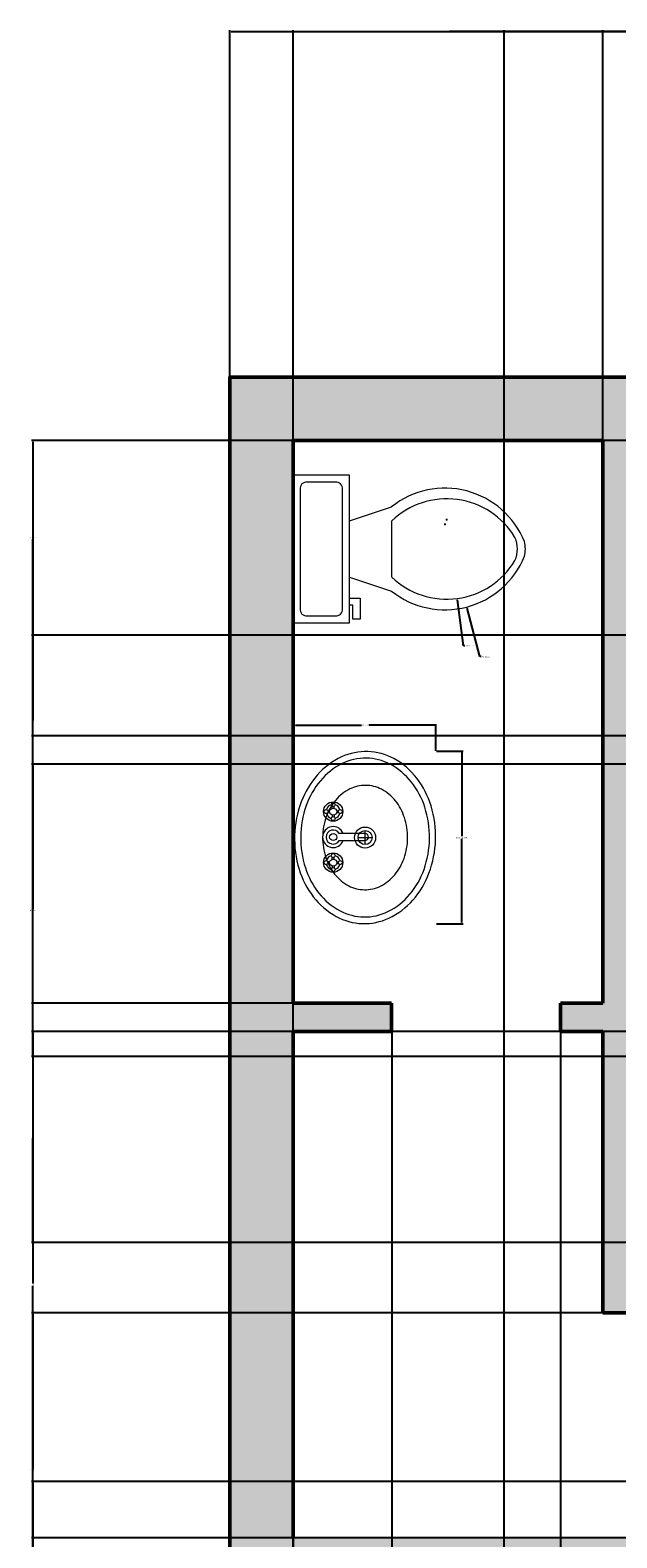
# Model space of a CAD drawing. Units: inches. Extents: x 1869 to 2483, y 2084 to 2479.
# Tile 3 of 7: x 1869 to 1952, y 2265 to 2479. Entities that reach past the tile are written whole.
import ezdxf

# ---------------------------------------------------------------- set-up
doc = ezdxf.new("R2010")
doc.units = ezdxf.units.IN
for name, color, linetype, lineweight in [('A-ANNO-DIMS', 2, 'Continuous', 18), ('A-FLOR-FIXT', 9, 'Continuous', 18), ('A-WALL', 7, 'Continuous', 50)]:
    doc.layers.add(name, color=color, linetype=linetype, lineweight=lineweight)
doc.layers.add('A-WALL-PATT', color=18, linetype='Continuous', lineweight=13, true_color=0x000000)
doc.styles.get("Standard").update_dxf_attribs({"font": 'arial.ttf'})
doc.dimstyles.get("Standard").update_dxf_attribs({"dimtxt": 0.18, "dimasz": 0.18, "dimexe": 0.18, "dimexo": 0.0625, "dimgap": 0.09, "dimtad": 0, "dimtih": 1, "dimtoh": 1, "dimdec": 4, "dimzin": 0, "dimdsep": 46, "dimtxsty": 'Standard', "dimcen": 0.09, "dimadec": 0, "dimazin": 0, "dimtfac": 1, "dimtdec": 4, "dimtofl": 0, "dimtmove": 0, "dimatfit": 3, "dimfxl": 1, "dimtolj": 1, "dimtzin": 0, "dimarcsym": 0})

# ---------------------------------------------------------------- blocks, each defined once
blk = doc.blocks.new('Toilet - top')
for p, q in [((9.5, -6), (9.5, -2)), ((-10, -8.5), (-8, -8.5)), ((-10, -9.5), (-10, -8.5)), ((-8, -8.5), (-8, -8)), ((-7, -8), (-7, -9.5)), ((-4, -8), (-6, -14)), ((4, -8), (6, -14)), ((-7, -9.5), (-10, -9.5)), ((4, -14), (-4, -14))]:
    blk.add_line(p, q)
blk.add_lwpolyline([(10.5, -8), (10.5, 0), (-10.5, 0), (-10.5, -8)], close=True)
for points in [[(-9.5, -2), (-9.5, -6)], [(8.5, -1), (-8.5, -1)], [(-8.5, -7), (8.5, -7)]]:
    blk.add_lwpolyline(points)
for centre, radius, start, end in [((-8.62, -1.88), 0.884, 81.8699, 188.1301), ((8.62, -1.88), 0.884, 351.8699, 98.1301), ((-8.62, -6.12), 0.884, 171.8699, 278.1301), ((8.62, -6.12), 0.884, 261.8699, 8.1301), ((3.52, -21.58), 12.17, 141.4691, 247.9714), ((4.2, -21.82), 11.33, 136.3677, 238.9468), ((-3.52, -21.58), 12.17, 292.0284, 38.5307), ((-4.2, -21.82), 11.33, 301.053, 43.6321), ((0, -27.88), 4, 245.7318, 294.2682), ((0, -29), 4, 254.8605, 285.1395)]:
    blk.add_arc(centre, radius, start, end)
blk = doc.blocks.new('Sink - Oval top')
for p, q in [((-1, 0), (1, 0)), ((0, 1), (0, -1))]:
    blk.add_line(p, q)
for points in [[(-12.23, 0.39, 0.117634), (-11.46, -3.36, 0.104469), (-8.88, -6.8, 0.090016), (-5.08, -9.07, 0.08192), (-0.32, -10.02, 0.08192), (4.49, -9.38, 0.090016), (8.42, -7.36, 0.104469), (11.22, -4.09, 0.117634), (12.23, -0.39, 0.117634), (11.46, 3.36, 0.104469), (8.88, 6.8, 0.090016), (5.08, 9.07, 0.08192), (0.32, 10.02, 0.08192), (-4.49, 9.38, 0.090016), (-8.42, 7.36, 0.104469), (-11.22, 4.09, 0.117634)], [(-11.29, 0.16, 0.118622), (-10.52, -3.25, 0.104678), (-8.07, -6.36, 0.089562), (-4.54, -8.37, 0.081185), (-0.13, -9.15, 0.081185), (4.3, -8.49, 0.089562), (7.89, -6.58, 0.104678), (10.42, -3.55, 0.118622), (11.29, -0.16, 0.118622), (10.52, 3.25, 0.104678), (8.07, 6.36, 0.089562), (4.54, 8.37, 0.081185), (0.13, 9.15, 0.081185), (-4.3, 8.49, 0.089562), (-7.89, 6.58, 0.104678), (-10.42, 3.55, 0.118622)], [(-7.42, 0.08, 0.118283), (-6.91, -2.17, 0.104607), (-5.29, -4.21, 0.089718), (-2.97, -5.53, 0.081436), (-0.07, -6.04, 0.081436), (2.84, -5.59, 0.089718), (5.2, -4.33, 0.104607), (6.86, -2.32, 0.118283), (7.42, -0.08, 0.118283), (6.91, 2.17, 0.104607), (5.29, 4.21, 0.089718), (2.97, 5.53, 0.081436), (0.07, 6.04, 0.081436), (-2.84, 5.59, 0.089718), (-5.2, 4.33, 0.104607), (-6.86, 2.32, 0.118283)]]:
    blk.add_lwpolyline(points, format="xyb", close=True)
for radius in [1.5, 1]:
    blk.add_circle((0, 0), radius)
blk = doc.blocks.new('Faucet - Bathroom top')
for p, q in [((-4.107, 0.125), (-4.375, 0.125)), ((-3.75, 0.4788), (-3.75, 0.75)), ((-3.5, 0.482), (-3.5, 0.75)), ((-3.1461, 0.125), (-2.875, 0.125)), ((3.143, 0.125), (2.875, 0.125)), ((3.5, 0.4788), (3.5, 0.75)), ((3.75, 0.482), (3.75, 0.75)), ((4.1039, 0.125), (4.375, 0.125)), ((-4.1039, -0.125), (-4.375, -0.125)), ((-3.75, -0.4821), (-3.75, -0.75)), ((-3.5, -0.4789), (-3.5, -0.75)), ((-3.143, -0.125), (-2.875, -0.125)), ((-0.5, -0.8639), (-0.5, -4.5)), ((0.5, -4.5), (0.5, -0.8631)), ((3.1461, -0.125), (2.875, -0.125)), ((3.5, -0.4821), (3.5, -0.75)), ((3.75, -0.4789), (3.75, -0.75)), ((4.107, -0.125), (4.375, -0.125))]:
    blk.add_line(p, q)
for centre, radius in [((-3.625, 0), 1.375), ((-4.625, 0), 0.2795), ((-3.625, 0), 0.5), ((-3.625, 1), 0.2795), ((-2.625, 0), 0.2795), ((0, 0), 0.5), ((3.625, 0), 1.375), ((2.625, 0), 0.2795), ((3.625, 0), 0.5), ((3.625, 1), 0.2795), ((4.625, 0), 0.2795), ((-3.625, -1), 0.2795), ((3.625, -1), 0.2795)]:
    blk.add_circle(centre, radius)
for centre, radius, start, end in [((-3.625, 0), 1, 105.2407, 164.2093), ((-3.625, 0), 1, 16.44125, 74.07887), ((0, 0), 1.5, 289.6514, 250.3603), ((0, 0), 1, 300.3431, 239.7554), ((3.625, 0), 1, 106.12, 164.0884), ((3.625, 0), 1, 16.23422, 73.90469), ((-3.625, 0), 1, 196.2342, 253.9047), ((-3.625, 0), 1, 286.12, 344.0884), ((3.625, 0), 1, 196.4413, 254.0789), ((3.625, 0), 1, 285.2407, 344.2093), ((0, -4.5), 0.5, 180, 0)]:
    blk.add_arc(centre, radius, start, end)
blk = doc.blocks.new('*D21')
at = {"layer": 'A-ANNO-DIMS', "color": 0, "lineweight": -2, "transparency": 16777216}
for p, q in [((1926.44, 2376.56), (1930.24, 2376.56)), ((1930.06, 2376.38), (1930.06, 2364.47)), ((1930.06, 2352.19), (1930.06, 2364.1)), ((1926.44, 2352.01), (1930.24, 2352.01))]:
    blk.add_line(p, q, dxfattribs=at)
at = {"layer": 'A-ANNO-DIMS', "color": 0, "transparency": 16777216}
for points in [[(1930.03, 2376.38), (1930.09, 2376.38), (1930.06, 2376.56)], [(1930.03, 2352.19), (1930.09, 2352.19), (1930.06, 2352.01)]]:
    blk.add_solid(points, dxfattribs=at)
at = {"layer": 'Defpoints', "color": 0, "transparency": 16777216}
for p in [(1926.37, 2376.56), (1930.06, 2376.56), (1926.37, 2352.01)]:
    blk.add_point(p, dxfattribs=at)
at = {"layer": 'A-ANNO-DIMS', "color": 0, "transparency": 16777216, "insert": (1930.06, 2364.28), "char_height": 0.18, "attachment_point": 5}
blk.add_mtext('\\A1;BASIN 25 TYP.', dxfattribs=at)
blk = doc.blocks.new('*D22')
at = {"layer": 'A-ANNO-DIMS', "color": 0, "lineweight": -2, "transparency": 16777216}
for p, q in [((1906.24, 2376.62), (1906.24, 2380.42)), ((1906.42, 2380.24), (1915.78, 2380.24)), ((1926.19, 2380.24), (1916.83, 2380.24)), ((1926.37, 2376.62), (1926.37, 2380.42))]:
    blk.add_line(p, q, dxfattribs=at)
at = {"layer": 'A-ANNO-DIMS', "color": 0, "transparency": 16777216}
for points in [[(1906.42, 2380.27), (1906.42, 2380.21), (1906.24, 2380.24)], [(1926.19, 2380.27), (1926.19, 2380.21), (1926.37, 2380.24)]]:
    blk.add_solid(points, dxfattribs=at)
at = {"layer": 'Defpoints', "color": 0, "transparency": 16777216}
for p in [(1906.24, 2380.24), (1906.24, 2376.56), (1926.37, 2376.56)]:
    blk.add_point(p, dxfattribs=at)
at = {"layer": 'A-ANNO-DIMS', "color": 0, "transparency": 16777216, "insert": (1916.31, 2380.24), "char_height": 0.18, "attachment_point": 5}
blk.add_mtext('\\A1;20 TYP.', dxfattribs=at)
blk = doc.blocks.new('*D35')
at = {"layer": 'A-ANNO-DIMS', "color": 0, "lineweight": -2, "transparency": 16777216}
for p, q in [((1906.08, 2420.79), (1906.08, 2479.07)), ((1906.26, 2478.89), (1927.86, 2478.89)), ((1949.9, 2478.89), (1928.3, 2478.89)), ((1950.08, 2420.79), (1950.08, 2479.07))]:
    blk.add_line(p, q, dxfattribs=at)
at = {"layer": 'A-ANNO-DIMS', "color": 0, "transparency": 16777216}
for points in [[(1906.26, 2478.92), (1906.26, 2478.86), (1906.08, 2478.89)], [(1949.9, 2478.92), (1949.9, 2478.86), (1950.08, 2478.89)]]:
    blk.add_solid(points, dxfattribs=at)
at = {"layer": 'Defpoints', "color": 0, "transparency": 16777216}
for p in [(1950.08, 2478.89), (1906.08, 2420.72), (1950.08, 2420.72)]:
    blk.add_point(p, dxfattribs=at)
at = {"layer": 'A-ANNO-DIMS', "color": 0, "transparency": 16777216, "insert": (1928.08, 2478.89), "char_height": 0.18, "attachment_point": 5}
blk.add_mtext('\\A1;44', dxfattribs=at)
blk = doc.blocks.new('*D45')
at = {"layer": 'A-ANNO-DIMS', "color": 0, "lineweight": -2, "transparency": 16777216}
for p, q in [((1906.02, 2336.72), (1868.9, 2336.72)), ((1869.08, 2336.54), (1869.08, 2300.9)), ((1869.08, 2264.9), (1869.08, 2300.54)), ((1906.02, 2264.72), (1868.9, 2264.72))]:
    blk.add_line(p, q, dxfattribs=at)
at = {"layer": 'A-ANNO-DIMS', "color": 0, "transparency": 16777216}
for points in [[(1869.05, 2336.54), (1869.11, 2336.54), (1869.08, 2336.72)], [(1869.05, 2264.9), (1869.11, 2264.9), (1869.08, 2264.72)]]:
    blk.add_solid(points, dxfattribs=at)
at = {"layer": 'Defpoints', "color": 0, "transparency": 16777216}
for p in [(1869.08, 2336.72), (1906.08, 2336.72), (1906.08, 2264.72)]:
    blk.add_point(p, dxfattribs=at)
at = {"layer": 'A-ANNO-DIMS', "color": 0, "transparency": 16777216, "insert": (1869.08, 2300.72), "char_height": 0.18, "attachment_point": 5}
blk.add_mtext('\\A1;72', dxfattribs=at)
blk = doc.blocks.new('*D46')
at = {"layer": 'A-ANNO-DIMS', "color": 0, "lineweight": -2, "transparency": 16777216}
for p, q in [((1906.02, 2420.72), (1868.9, 2420.72)), ((1869.08, 2420.54), (1869.08, 2380.91)), ((1869.08, 2340.9), (1869.08, 2380.54)), ((1906.02, 2340.72), (1868.9, 2340.72))]:
    blk.add_line(p, q, dxfattribs=at)
at = {"layer": 'A-ANNO-DIMS', "color": 0, "transparency": 16777216}
for points in [[(1869.05, 2420.54), (1869.11, 2420.54), (1869.08, 2420.72)], [(1869.05, 2340.9), (1869.11, 2340.9), (1869.08, 2340.72)]]:
    blk.add_solid(points, dxfattribs=at)
at = {"layer": 'Defpoints', "color": 0, "transparency": 16777216}
for p in [(1869.08, 2420.72), (1906.08, 2420.72), (1906.08, 2340.72)]:
    blk.add_point(p, dxfattribs=at)
at = {"layer": 'A-ANNO-DIMS', "color": 0, "transparency": 16777216, "insert": (1869.08, 2380.72), "char_height": 0.18, "attachment_point": 5}
blk.add_mtext('\\A1;80', dxfattribs=at)
blk = doc.blocks.new('*D47')
at = {"layer": 'A-ANNO-DIMS', "color": 0, "lineweight": -2, "transparency": 16777216}
for p, q in [((2322.02, 2420.72), (1868.9, 2420.72)), ((1869.08, 2420.54), (1869.08, 2399.9)), ((1869.08, 2378.9), (1869.08, 2399.54)), ((2322.02, 2378.72), (1868.9, 2378.72))]:
    blk.add_line(p, q, dxfattribs=at)
at = {"layer": 'A-ANNO-DIMS', "color": 0, "transparency": 16777216}
for points in [[(1869.05, 2420.54), (1869.11, 2420.54), (1869.08, 2420.72)], [(1869.05, 2378.9), (1869.11, 2378.9), (1869.08, 2378.72)]]:
    blk.add_solid(points, dxfattribs=at)
at = {"layer": 'Defpoints', "color": 0, "transparency": 16777216}
for p in [(1869.08, 2420.72), (2322.08, 2420.72), (2322.08, 2378.72)]:
    blk.add_point(p, dxfattribs=at)
at = {"layer": 'A-ANNO-DIMS', "color": 0, "transparency": 16777216, "insert": (1869.08, 2399.72), "char_height": 0.18, "attachment_point": 5}
blk.add_mtext('\\A1;42', dxfattribs=at)
blk = doc.blocks.new('*D49')
at = {"layer": 'A-ANNO-DIMS', "color": 0, "lineweight": -2, "transparency": 16777216}
for p, q in [((1906.08, 2260.79), (1906.08, 2479.07)), ((1906.26, 2478.89), (1935.86, 2478.89)), ((1965.9, 2478.89), (1936.3, 2478.89)), ((1966.08, 2260.79), (1966.08, 2479.07))]:
    blk.add_line(p, q, dxfattribs=at)
at = {"layer": 'A-ANNO-DIMS', "color": 0, "transparency": 16777216}
for points in [[(1906.26, 2478.92), (1906.26, 2478.86), (1906.08, 2478.89)], [(1965.9, 2478.92), (1965.9, 2478.86), (1966.08, 2478.89)]]:
    blk.add_solid(points, dxfattribs=at)
at = {"layer": 'Defpoints', "color": 0, "transparency": 16777216}
for p in [(1966.08, 2478.89), (1906.08, 2260.72), (1966.08, 2260.72)]:
    blk.add_point(p, dxfattribs=at)
at = {"layer": 'A-ANNO-DIMS', "color": 0, "transparency": 16777216, "insert": (1936.08, 2478.89), "char_height": 0.18, "attachment_point": 5}
blk.add_mtext('\\A1;60', dxfattribs=at)
blk = doc.blocks.new('*D57')
at = {"layer": 'A-ANNO-DIMS', "color": 0, "lineweight": -2, "transparency": 16777216}
for p, q in [((2446.02, 2296.72), (1868.9, 2296.72)), ((1869.08, 2296.54), (1869.08, 2274.58)), ((1869.08, 2252.25), (1869.08, 2274.22)), ((2446.02, 2252.07), (1868.9, 2252.07))]:
    blk.add_line(p, q, dxfattribs=at)
at = {"layer": 'A-ANNO-DIMS', "color": 0, "transparency": 16777216}
for points in [[(1869.05, 2296.54), (1869.11, 2296.54), (1869.08, 2296.72)], [(1869.05, 2252.25), (1869.11, 2252.25), (1869.08, 2252.07)]]:
    blk.add_solid(points, dxfattribs=at)
at = {"layer": 'Defpoints', "color": 0, "transparency": 16777216}
for p in [(1869.08, 2296.72), (2446.08, 2296.72), (2446.08, 2252.07)]:
    blk.add_point(p, dxfattribs=at)
at = {"layer": 'A-ANNO-DIMS', "color": 0, "transparency": 16777216, "insert": (1869.08, 2274.4), "char_height": 0.18, "attachment_point": 5}
blk.add_mtext('\\A1;44.65', dxfattribs=at)
blk = doc.blocks.new('*D62')
at = {"layer": 'A-ANNO-DIMS', "color": 0, "lineweight": -2, "transparency": 16777216}
for p, q in [((2322.02, 2336.72), (1868.9, 2336.72)), ((1869.08, 2336.54), (1869.08, 2321.91)), ((1869.08, 2306.9), (1869.08, 2321.54)), ((2322.02, 2306.72), (1868.9, 2306.72))]:
    blk.add_line(p, q, dxfattribs=at)
at = {"layer": 'A-ANNO-DIMS', "color": 0, "transparency": 16777216}
for points in [[(1869.05, 2336.54), (1869.11, 2336.54), (1869.08, 2336.72)], [(1869.05, 2306.9), (1869.11, 2306.9), (1869.08, 2306.72)]]:
    blk.add_solid(points, dxfattribs=at)
at = {"layer": 'Defpoints', "color": 0, "transparency": 16777216}
for p in [(1869.08, 2336.72), (2322.08, 2336.72), (2322.08, 2306.72)]:
    blk.add_point(p, dxfattribs=at)
at = {"layer": 'A-ANNO-DIMS', "color": 0, "transparency": 16777216, "insert": (1869.08, 2321.72), "char_height": 0.18, "attachment_point": 5}
blk.add_mtext('\\A1;30', dxfattribs=at)
blk = doc.blocks.new('*D63')
at = {"layer": 'A-ANNO-DIMS', "color": 0, "lineweight": -2, "transparency": 16777216}
for p, q in [((2348.34, 2272.72), (1868.9, 2272.72)), ((1869.08, 2272.54), (1869.08, 2257.91)), ((1869.08, 2242.9), (1869.08, 2257.54)), ((2348.34, 2242.72), (1868.9, 2242.72))]:
    blk.add_line(p, q, dxfattribs=at)
at = {"layer": 'A-ANNO-DIMS', "color": 0, "transparency": 16777216}
for points in [[(1869.05, 2272.54), (1869.11, 2272.54), (1869.08, 2272.72)], [(1869.05, 2242.9), (1869.11, 2242.9), (1869.08, 2242.72)]]:
    blk.add_solid(points, dxfattribs=at)
at = {"layer": 'Defpoints', "color": 0, "transparency": 16777216}
for p in [(1869.08, 2272.72), (2348.4, 2272.72), (2348.4, 2242.72)]:
    blk.add_point(p, dxfattribs=at)
at = {"layer": 'A-ANNO-DIMS', "color": 0, "transparency": 16777216, "insert": (1869.08, 2257.72), "char_height": 0.18, "attachment_point": 5}
blk.add_mtext('\\A1;30', dxfattribs=at)
blk = doc.blocks.new('*D67')
at = {"layer": 'A-ANNO-DIMS', "color": 0, "lineweight": -2, "transparency": 16777216}
for p, q in [((1936.08, 2216.79), (1936.08, 2479.07)), ((1936.26, 2478.89), (1947.86, 2478.89)), ((1959.9, 2478.89), (1948.3, 2478.89)), ((1960.08, 2216.79), (1960.08, 2479.07))]:
    blk.add_line(p, q, dxfattribs=at)
at = {"layer": 'A-ANNO-DIMS', "color": 0, "transparency": 16777216}
for points in [[(1936.26, 2478.92), (1936.26, 2478.86), (1936.08, 2478.89)], [(1959.9, 2478.92), (1959.9, 2478.86), (1960.08, 2478.89)]]:
    blk.add_solid(points, dxfattribs=at)
at = {"layer": 'Defpoints', "color": 0, "transparency": 16777216}
for p in [(1960.08, 2478.89), (1936.08, 2216.72), (1960.08, 2216.72)]:
    blk.add_point(p, dxfattribs=at)
at = {"layer": 'A-ANNO-DIMS', "color": 0, "transparency": 16777216, "insert": (1948.08, 2478.89), "char_height": 0.18, "attachment_point": 5}
blk.add_mtext('\\A1;24', dxfattribs=at)
blk = doc.blocks.new('*D69')
at = {"layer": 'A-ANNO-DIMS', "color": 0, "lineweight": -2, "transparency": 16777216}
for p, q in [((1920.08, 2336.66), (1920.08, 2083.54)), ((1944.08, 2336.66), (1944.08, 2083.54)), ((1920.26, 2083.72), (1931.86, 2083.72)), ((1943.9, 2083.72), (1932.3, 2083.72))]:
    blk.add_line(p, q, dxfattribs=at)
at = {"layer": 'A-ANNO-DIMS', "color": 0, "transparency": 16777216}
for points in [[(1920.26, 2083.75), (1920.26, 2083.69), (1920.08, 2083.72)], [(1943.9, 2083.75), (1943.9, 2083.69), (1944.08, 2083.72)]]:
    blk.add_solid(points, dxfattribs=at)
at = {"layer": 'Defpoints', "color": 0, "transparency": 16777216}
for p in [(1920.08, 2336.72), (1944.08, 2336.72), (1944.08, 2083.72)]:
    blk.add_point(p, dxfattribs=at)
at = {"layer": 'A-ANNO-DIMS', "color": 0, "transparency": 16777216, "insert": (1932.08, 2083.72), "char_height": 0.18, "attachment_point": 5}
blk.add_mtext('\\A1;24', dxfattribs=at)
blk = doc.blocks.new('*D74')
at = {"layer": 'A-ANNO-DIMS', "color": 0, "lineweight": -2, "transparency": 16777216}
for p, q in [((1950.02, 2296.72), (1868.9, 2296.72)), ((1869.08, 2296.54), (1869.08, 2280.91)), ((1869.08, 2264.9), (1869.08, 2280.54)), ((2010.02, 2264.72), (1868.9, 2264.72))]:
    blk.add_line(p, q, dxfattribs=at)
at = {"layer": 'A-ANNO-DIMS', "color": 0, "transparency": 16777216}
for points in [[(1869.05, 2296.54), (1869.11, 2296.54), (1869.08, 2296.72)], [(1869.05, 2264.9), (1869.11, 2264.9), (1869.08, 2264.72)]]:
    blk.add_solid(points, dxfattribs=at)
at = {"layer": 'Defpoints', "color": 0, "transparency": 16777216}
for p in [(1869.08, 2296.72), (1950.08, 2296.72), (2010.08, 2264.72)]:
    blk.add_point(p, dxfattribs=at)
at = {"layer": 'A-ANNO-DIMS', "color": 0, "transparency": 16777216, "insert": (1869.08, 2280.72), "char_height": 0.18, "attachment_point": 5}
blk.add_mtext('\\A1;32', dxfattribs=at)
blk = doc.blocks.new('*D75')
at = {"layer": 'A-ANNO-DIMS', "color": 0, "lineweight": -2, "transparency": 16777216}
for p, q in [((1897.08, 2429.79), (1897.08, 2479.07)), ((1897.26, 2478.89), (2175.79, 2478.89)), ((2454.9, 2478.89), (2176.37, 2478.89)), ((2455.08, 2429.79), (2455.08, 2479.07))]:
    blk.add_line(p, q, dxfattribs=at)
at = {"layer": 'A-ANNO-DIMS', "color": 0, "transparency": 16777216}
for points in [[(1897.26, 2478.92), (1897.26, 2478.86), (1897.08, 2478.89)], [(2454.9, 2478.92), (2454.9, 2478.86), (2455.08, 2478.89)]]:
    blk.add_solid(points, dxfattribs=at)
at = {"layer": 'Defpoints', "color": 0, "transparency": 16777216}
for p in [(2455.08, 2478.89), (1897.08, 2429.72), (2455.08, 2429.72)]:
    blk.add_point(p, dxfattribs=at)
at = {"layer": 'A-ANNO-DIMS', "color": 0, "transparency": 16777216, "insert": (2176.08, 2478.89), "char_height": 0.18, "attachment_point": 5}
blk.add_mtext('\\A1;558', dxfattribs=at)
blk = doc.blocks.new('*D84')
at = {"layer": 'A-ANNO-DIMS', "color": 0, "lineweight": -2, "transparency": 16777216}
for p, q in [((1906.08, 2336.66), (1906.08, 2083.54)), ((1920.08, 2336.66), (1920.08, 2083.54)), ((1906.26, 2083.72), (1912.87, 2083.72)), ((1919.9, 2083.72), (1913.29, 2083.72))]:
    blk.add_line(p, q, dxfattribs=at)
at = {"layer": 'A-ANNO-DIMS', "color": 0, "transparency": 16777216}
for points in [[(1906.26, 2083.75), (1906.26, 2083.69), (1906.08, 2083.72)], [(1919.9, 2083.75), (1919.9, 2083.69), (1920.08, 2083.72)]]:
    blk.add_solid(points, dxfattribs=at)
at = {"layer": 'Defpoints', "color": 0, "transparency": 16777216}
for p in [(1906.08, 2336.72), (1920.08, 2336.72), (1920.08, 2083.72)]:
    blk.add_point(p, dxfattribs=at)
at = {"layer": 'A-ANNO-DIMS', "color": 0, "transparency": 16777216, "insert": (1913.08, 2083.72), "char_height": 0.18, "attachment_point": 5}
blk.add_mtext('\\A1;14', dxfattribs=at)
blk = doc.blocks.new('*D94')
at = {"layer": 'A-ANNO-DIMS', "color": 0, "lineweight": -2, "transparency": 16777216}
for p, q in [((2170.02, 2374.72), (1868.9, 2374.72)), ((1869.08, 2374.54), (1869.08, 2354.12)), ((1869.08, 2333.33), (1869.08, 2353.75)), ((2180.87, 2333.15), (1868.9, 2333.15))]:
    blk.add_line(p, q, dxfattribs=at)
at = {"layer": 'A-ANNO-DIMS', "color": 0, "transparency": 16777216}
for points in [[(1869.05, 2374.54), (1869.11, 2374.54), (1869.08, 2374.72)], [(1869.05, 2333.33), (1869.11, 2333.33), (1869.08, 2333.15)]]:
    blk.add_solid(points, dxfattribs=at)
at = {"layer": 'Defpoints', "color": 0, "transparency": 16777216}
for p in [(2170.08, 2374.72), (1869.08, 2333.15), (2180.94, 2333.15)]:
    blk.add_point(p, dxfattribs=at)
at = {"layer": 'A-ANNO-DIMS', "color": 0, "transparency": 16777216, "insert": (1869.08, 2353.94), "char_height": 0.18, "attachment_point": 5}
blk.add_mtext('\\A1;41.575', dxfattribs=at)
blk = doc.blocks.new('*D96')
at = {"layer": 'A-ANNO-DIMS', "color": 0, "lineweight": -2, "transparency": 16777216}
for p, q in [((2446.02, 2420.72), (1868.9, 2420.72)), ((1869.08, 2420.54), (1869.08, 2407.07)), ((1869.08, 2393.24), (1869.08, 2406.71)), ((2446.08, 2393.06), (1868.9, 2393.06))]:
    blk.add_line(p, q, dxfattribs=at)
at = {"layer": 'A-ANNO-DIMS', "color": 0, "transparency": 16777216}
for points in [[(1869.05, 2420.54), (1869.11, 2420.54), (1869.08, 2420.72)], [(1869.05, 2393.24), (1869.11, 2393.24), (1869.08, 2393.06)]]:
    blk.add_solid(points, dxfattribs=at)
at = {"layer": 'Defpoints', "color": 0, "transparency": 16777216}
for p in [(1869.08, 2420.72), (2446.08, 2420.72), (2446.14, 2393.06)]:
    blk.add_point(p, dxfattribs=at)
at = {"layer": 'A-ANNO-DIMS', "color": 0, "transparency": 16777216, "insert": (1869.08, 2406.89), "char_height": 0.18, "attachment_point": 5}
blk.add_mtext('\\A1;27.667', dxfattribs=at)
blk = doc.blocks.new('*D98')
at = {"layer": 'A-ANNO-DIMS', "color": 0, "lineweight": -2, "transparency": 16777216}
for p, q in [((1927.57, 2408.83), (1927.75, 2408.83)), ((1927.66, 2408.74), (1927.66, 2408.92)), ((1932.61, 2390), (1930.8, 2396.88)), ((1932.79, 2390), (1932.61, 2390))]:
    blk.add_line(p, q, dxfattribs=at)
at = {"layer": 'A-ANNO-DIMS', "color": 0, "transparency": 16777216}
blk.add_solid([(1930.83, 2396.89), (1930.77, 2396.88), (1930.75, 2397.06)], dxfattribs=at)
at = {"layer": 'Defpoints', "color": 0, "transparency": 16777216}
for p in [(1927.66, 2408.83), (1930.75, 2397.06)]:
    blk.add_point(p, dxfattribs=at)
at = {"layer": 'A-ANNO-DIMS', "color": 0, "transparency": 16777216, "insert": (1933.47, 2390), "char_height": 0.18, "attachment_point": 5}
blk.add_mtext('\\A1;4X R12.17', dxfattribs=at)
blk = doc.blocks.new('*D99')
at = {"layer": 'A-ANNO-DIMS', "color": 0, "lineweight": -2, "transparency": 16777216}
for p, q in [((1927.81, 2409.51), (1927.99, 2409.51)), ((1927.9, 2409.42), (1927.9, 2409.6)), ((1930.31, 2391.54), (1929.43, 2398.1)), ((1930.49, 2391.54), (1930.31, 2391.54))]:
    blk.add_line(p, q, dxfattribs=at)
at = {"layer": 'A-ANNO-DIMS', "color": 0, "transparency": 16777216}
blk.add_solid([(1929.46, 2398.1), (1929.4, 2398.1), (1929.41, 2398.28)], dxfattribs=at)
at = {"layer": 'Defpoints', "color": 0, "transparency": 16777216}
for p in [(1927.9, 2409.51), (1929.41, 2398.28)]:
    blk.add_point(p, dxfattribs=at)
at = {"layer": 'A-ANNO-DIMS', "color": 0, "transparency": 16777216, "insert": (1931.17, 2391.54), "char_height": 0.18, "attachment_point": 5}
blk.add_mtext('\\A1;4X R11.33', dxfattribs=at)

msp = doc.modelspace()

# ---------------------------------------------------------------- hatches: boundary and pattern name
at = {"layer": 'A-WALL-PATT'}
h = msp.add_hatch(color=256, dxfattribs=at)
h.dxf.hatch_style = 1
h.paths.add_polyline_path([(1998.5221, 2429.7235), (1897.0799, 2429.7235), (1897.0799, 2252.2488), (1906.0799, 2252.2488), (1906.0799, 2260.7235), (1966.0799, 2260.7235), (1966.0799, 2216.7235), (1960.0791, 2216.7235), (1960.0161, 2212.7235), (2050.0707, 2212.7235), (2050.1612, 2216.7235), (2010.0799, 2216.7235), (2010.0799, 2226.7235), (2006.0799, 2226.7235), (2006.0799, 2216.7235), (1970.0799, 2216.7235), (1970.0799, 2260.7235), (2006.0799, 2260.7235), (2006.0799, 2250.7235), (2010.0799, 2250.7235), (2010.0799, 2264.7235), (1906.0799, 2264.7235), (1906.0799, 2336.7235), (1920.0799, 2336.7235), (1920.0799, 2340.7235), (1906.0799, 2340.7235), (1906.0799, 2420.7235), (1950.0799, 2420.7235), (1950.0799, 2340.7235), (1944.0799, 2340.7235), (1944.0799, 2336.7235), (1950.0799, 2336.7235), (1950.0799, 2296.7235), (2050.0799, 2296.7235), (2050.0799, 2300.7235), (1954.0799, 2300.7235), (1954.0799, 2420.7235), (1998.5221, 2420.7235)])

# ---------------------------------------------------------------- linework, layer by layer
at = {"layer": 'A-WALL'}
for p, q in [((1906.0799, 2420.7235), (1950.0799, 2420.7235)), ((1906.0799, 2340.7235), (1906.0799, 2420.7235)), ((1950.0799, 2340.7235), (1950.0799, 2420.7235)), ((1906.0799, 2340.7235), (1920.0799, 2340.7235)), ((1920.0799, 2340.7235), (1920.0799, 2336.7235)), ((1944.0799, 2340.7235), (1944.0799, 2336.7235)), ((1944.0799, 2340.7235), (1950.0799, 2340.7235)), ((1906.0799, 2300.7235), (1906.0799, 2336.7235)), ((1906.0799, 2264.7235), (1906.0799, 2336.7235)), ((1906.0799, 2336.7235), (1920.0799, 2336.7235)), ((1944.0799, 2336.7235), (1950.0799, 2336.7235)), ((1950.0799, 2296.7235), (1950.0799, 2336.7235)), ((1950.0799, 2296.7235), (2050.0799, 2296.7235))]:
    msp.add_line(p, q, dxfattribs=at)
msp.add_lwpolyline([(2152.0799, 2111.7235), (1897.0799, 2111.7235), (1897.0799, 2429.7235), (2455.0799, 2429.7235), (2455.0799, 2111.7235), (2200.0799, 2111.7235)], dxfattribs=at)

# ---------------------------------------------------------------- block references
at = {"layer": 'A-FLOR-FIXT', "rotation": 90}
for name, p in [('Toilet - top', (1906.0799, 2405.3069)), ('Sink - Oval top', (1916.3051, 2364.282)), ('Faucet - Bathroom top', (1911.7683, 2364.3496))]:
    msp.add_blockref(name, p, dxfattribs=at)

# ---------------------------------------------------------------- dimensions: what is measured, and where the dimension line sits
at = {"layer": 'A-ANNO-DIMS'}
for base, p1, p2, picture, middle in [((2455.0799, 2478.8871), (1897.0799, 2429.7235), (2455.0799, 2429.7235), '*D75', (2176.0799, 2478.8871)), ((1950.0799, 2478.8871), (1906.0799, 2420.7235), (1950.0799, 2420.7235), '*D35', (1928.0799, 2478.8871)), ((1966.0799, 2478.8871), (1906.0799, 2260.7235), (1966.0799, 2260.7235), '*D49', (1936.0799, 2478.8871)), ((1960.0791, 2478.8871), (1936.0791, 2216.7235), (1960.0791, 2216.7235), '*D67', (1948.0791, 2478.8871)), ((1920.0799, 2083.7235), (1906.0799, 2336.7235), (1920.0799, 2336.7235), '*D84', (1913.0799, 2083.7235)), ((1944.0799, 2083.7235), (1920.0799, 2336.7235), (1944.0799, 2336.7235), '*D69', (1932.0799, 2083.7235))]:
    dim = msp.add_linear_dim(base=base, p1=p1, p2=p2, dimstyle='Standard', override={"dimdec": 0, "dimlfac": 1, "dimrnd": 0, "dimzin": 0, "dimdsep": 46, "dimlunit": 2}, dxfattribs=at)
    dim.commit()
    dim.dimension.update_dxf_attribs({"geometry": picture, "text_midpoint": middle})
for base, p1, p2, override, picture, middle in [((1869.0799, 2420.7235), (2446.143, 2393.0569), (2446.0799, 2420.7235), {"dimdec": 3, "dimlfac": 1, "dimrnd": 0, "dimzin": 0, "dimdsep": 46, "dimlunit": 2}, '*D96', (1869.0799, 2406.8902)), ((1869.0799, 2420.7235), (1906.0799, 2340.7235), (1906.0799, 2420.7235), {"dimdec": 0, "dimlfac": 1, "dimrnd": 0, "dimzin": 0, "dimdsep": 46, "dimlunit": 2}, '*D46', (1869.0799, 2380.7235)), ((1869.0799, 2420.7235), (2322.0799, 2378.7235), (2322.0799, 2420.7235), {"dimdec": 0, "dimlfac": 1, "dimrnd": 0, "dimzin": 0, "dimdsep": 46, "dimlunit": 2}, '*D47', (1869.0799, 2399.7235)), ((1869.0799, 2333.1488), (2170.0799, 2374.7235), (2180.9372, 2333.1488), {"dimdec": 3, "dimlfac": 1, "dimrnd": 0, "dimzin": 0, "dimdsep": 46, "dimlunit": 2}, '*D94', (1869.0799, 2353.9361)), ((1869.0799, 2336.7235), (1906.0799, 2264.7235), (1906.0799, 2336.7235), {"dimdec": 0, "dimlfac": 1, "dimrnd": 0, "dimzin": 0, "dimdsep": 46, "dimlunit": 2}, '*D45', (1869.0799, 2300.7235)), ((1869.0799, 2336.7235), (2322.0799, 2306.7235), (2322.0799, 2336.7235), {"dimdec": 0, "dimlfac": 1, "dimrnd": 0, "dimzin": 0, "dimdsep": 46, "dimlunit": 2}, '*D62', (1869.0799, 2321.7235)), ((1869.0799, 2296.7235), (2446.0799, 2252.0706), (2446.0799, 2296.7235), {"dimdec": 2, "dimlfac": 1, "dimrnd": 0, "dimzin": 0, "dimdsep": 46, "dimlunit": 2}, '*D57', (1869.0799, 2274.3971)), ((1869.0799, 2296.7235), (2010.0799, 2264.7235), (1950.0799, 2296.7235), {"dimdec": 0, "dimlfac": 1, "dimrnd": 0, "dimzin": 0, "dimdsep": 46, "dimlunit": 2}, '*D74', (1869.0799, 2280.7235)), ((1869.0799, 2272.7235), (2348.3982, 2242.7235), (2348.3982, 2272.7235), {"dimdec": 0, "dimlfac": 1, "dimrnd": 0, "dimzin": 0, "dimdsep": 46, "dimlunit": 2}, '*D63', (1869.0799, 2257.7235))]:
    dim = msp.add_linear_dim(base=base, p1=p1, p2=p2, angle=90, dimstyle='Standard', override=override, dxfattribs=at)
    dim.commit()
    dim.dimension.update_dxf_attribs({"geometry": picture, "text_midpoint": middle})
for center, mpoint, picture, middle in [((1927.8973, 2409.5069), (1929.407, 2398.2787), '*D99', (1931.1697, 2391.5419)), ((1927.6604, 2408.8265), (1930.753, 2397.057), '*D98', (1933.4654, 2389.9953))]:
    dim = msp.add_radius_dim(center=center, mpoint=mpoint, text='4X <>', dimstyle='Standard', override={"dimdec": 2, "dimlfac": 1, "dimrnd": 0, "dimzin": 0, "dimdsep": 46, "dimlunit": 2}, dxfattribs=at)
    dim.commit()
    dim.dimension.update_dxf_attribs({"geometry": picture, "text_midpoint": middle, "dimtype": 164})
for base, p1, p2, angle, text, picture, middle in [((1906.2368, 2380.24), (1926.3734, 2376.5574), (1906.2368, 2376.5574), 180, '<> TYP.', '*D22', (1916.3051, 2380.24)), ((1930.0561, 2376.5574), (1926.3734, 2352.0065), (1926.3734, 2376.5574), 90, 'BASIN <> TYP.', '*D21', (1930.0561, 2364.282))]:
    dim = msp.add_linear_dim(base=base, p1=p1, p2=p2, angle=angle, text=text, dimstyle='Standard', override={"dimdec": 0, "dimlfac": 1, "dimrnd": 0, "dimzin": 0, "dimdsep": 46, "dimlunit": 2}, dxfattribs=at)
    dim.commit()
    dim.dimension.update_dxf_attribs({"geometry": picture, "text_midpoint": middle})

doc.saveas('drawing.dxf')
